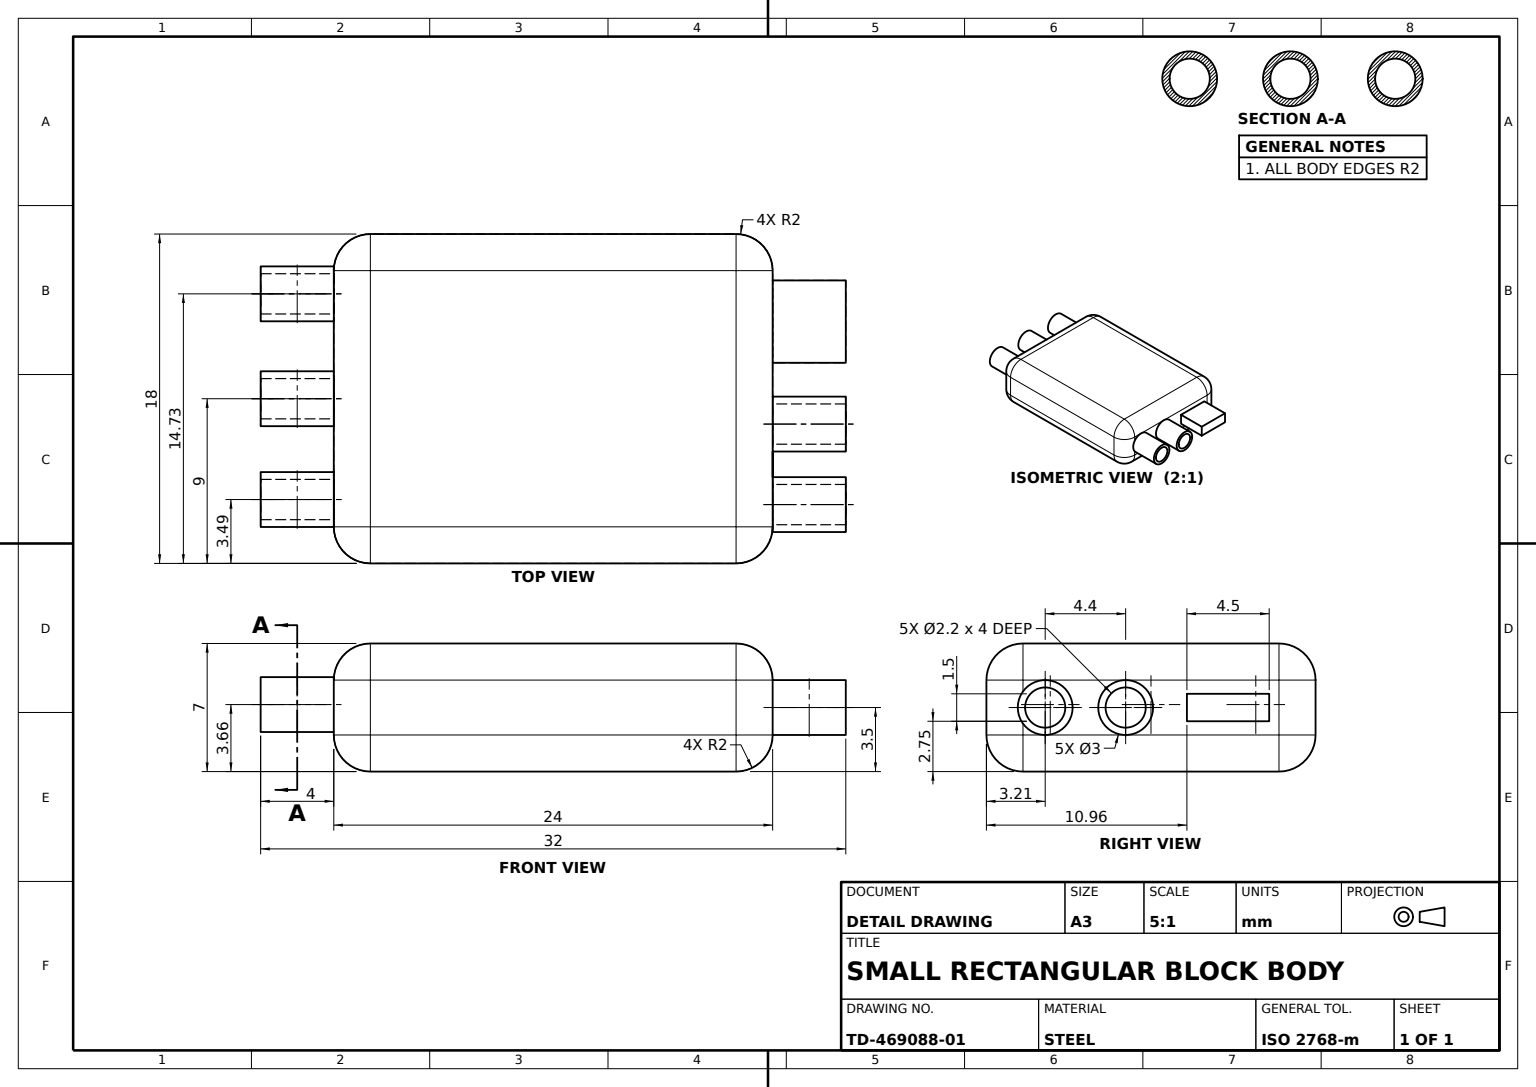
SolidWorks part; units mm, degrees
material "Plain Carbon Steel"
ref_plane "Front Plane" through (0, 0, 0) normal (0, 0, 1) x (1, 0, 0)
ref_plane "Top Plane" through (0, 0, 0) normal (0, 1, 0) x (1, 0, 0)
ref_plane "Right Plane" through (0, 0, 0) normal (1, 0, 0) x (0, 0, -1)
sketch "Housing Profile Sketch" plane through (0, 0, 0) normal (0, 1, 0) x (1, 0, 0)
  line L1 (-10, 9) -> (10, 9)
  line L2 (-12, 7) -> (-12, -7)
  line L3 (-10, -9) -> (10, -9)
  line L4 (12, 7) -> (12, -7)
  line L5 (-12, 9) -> (12, -9) construction
  line L6 (-12, -9) -> (12, 9) construction
  arc A0 (10, 9) -> (12, 7) centre (10, 7) cw
  arc A1 (10, -9) -> (12, -7) centre (10, -7) ccw
  arc A2 (-12, -7) -> (-10, -9) centre (-10, -7) ccw
  arc A3 (-10, 9) -> (-12, 7) centre (-10, 7) ccw
  point P0 (0, 0)
  dimension "D3" = 2
  dimension "D1" = 24
  dimension "D2" = 18
extrude "Housing Body" add sketch "Housing Profile Sketch" along normal blind 7
fillet "Housing Edge Fillet R2" radius 2 16 edges at (-11.4142, 0, 8.4142) (-12, 0, 0) (-11.4142, 0, -8.4142) (0, 0, -9) (11.4142, 0, -8.4142) (12, 0, 0) (11.4142, 0, 8.4142) (-11.4142, 7, 8.4142) (-12, 7, 0) (-11.4142, 7, -8.4142) (0, 7, -9) (11.4142, 7, -8.4142) (12, 7, 0) (11.4142, 7, 8.4142) (0, 0, 9) (0, 7, 9)
sketch "Pin Set A Sketch" plane through (-12, 0, 0) normal (-1, 0, 0) x (0, 0, 1)
  line L0 (-7, 5) -> (-7, 2) construction
  line L1 (-7, 3.6617) -> (7, 3.6617) construction
  line L2 (7, 5) -> (7, 2) construction
  line L3 (-7, 2) -> (7, 2) construction
  circle A0 centre (0, 3.6617) radius 1.5
  circle A1 centre (0, 3.6617) radius 1.1
  circle A2 centre (-5.7312, 3.6617) radius 1.5
  circle A3 centre (-5.7312, 3.6617) radius 1.1
  circle A4 centre (5.5088, 3.6617) radius 1.5
  circle A5 centre (5.5088, 3.6617) radius 1.1
  dimension "D1" = 3
  dimension "D2" = 0.4
  dimension "D3" = 1.2688
  dimension "D4" = 12.5088
  dimension "D5" = 1.6617
extrude "Tubular Pins Set A Ø3" add sketch "Pin Set A Sketch" along normal blind 4
sketch "Pin Set B and Tab Sketch" plane through (12, 0, 0) normal (1, 0, 0) x (0, 0, -1)
  line L0 (-7, 3.5) -> (7, 3.5) construction
  line L1 (-7, 5) -> (-7, 2) construction
  line L2 (7, 5) -> (7, 2) construction
  line L4 (1.9643, 2.75) -> (6.4643, 2.75)
  line L5 (1.9643, 2.75) -> (1.9643, 4.25)
  line L6 (1.9643, 4.25) -> (6.4643, 4.25)
  line L7 (6.4643, 2.75) -> (6.4643, 4.25)
  circle A0 centre (-5.7853, 3.5) radius 1.5
  circle A1 centre (-1.3853, 3.5) radius 1.5
  circle A2 centre (-5.7853, 3.5) radius 1.1
  circle A3 centre (-1.3853, 3.5) radius 1.1
  dimension "D3" = 3
  dimension "D4" = 0.4
  dimension "D5" = 4.4
  dimension "D6" = 1.2147
  dimension "D7" = 8.9643
  dimension "D1" = 4.5
  dimension "D2" = 1.5
extrude "Tubular Pins Set B and Tab" add sketch "Pin Set B and Tab Sketch" along normal blind 4
